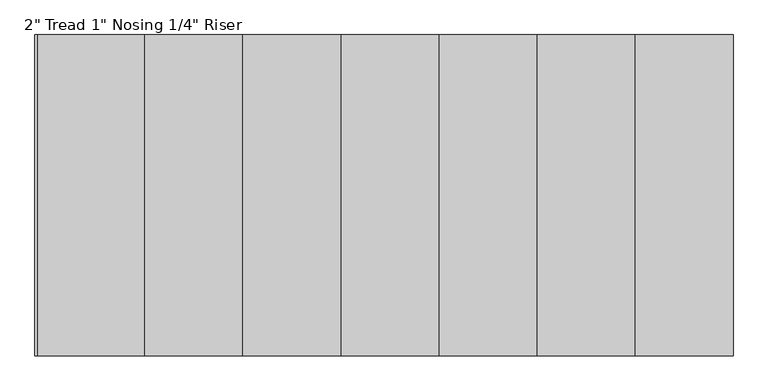
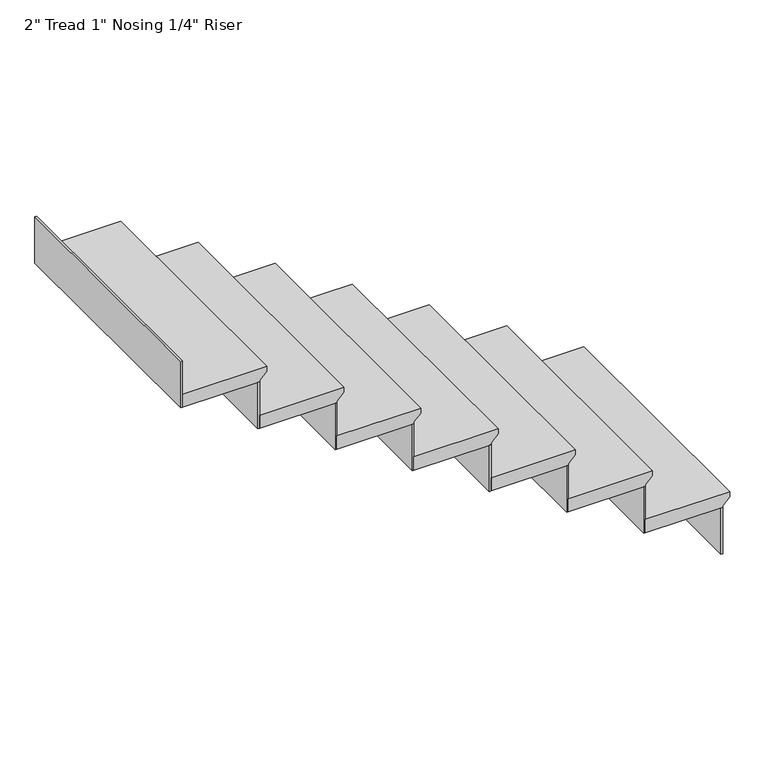
"""IFC4 building model written with IfcOpenShell, lengths in millimetres: stair flight geometry."""

from ifc_helpers import new_model, si_unit, frame, origin, place, context, project, spatial, polyline, outline, extrude, source, transform, mapped, element, save


def stair_flight_9d522be5(model_context):
    return source(origin(), model_context, "Body", "SweptSolid", [
        extrude(outline(polyline([(2565.4, -2377.5918815), (2565.4, -2682.3918815), (2514.6, -2682.3918815), (2514.6, -2402.9918815), (2520.95, -2402.9918815), (2546.35, -2377.5918815), (2565.4, -2377.5918815)])), frame((0.0, 1719.6168074, 0.0), z_axis=(0.0, 1.0, 0.0), x_axis=(0.0, 0.0, 1.0)), (0.0, 0.0, 1.0), 914.4),
        extrude(outline(polyline([(-2409.3418815, 2634.0168074), (-2402.9918815, 2634.0168074), (-2402.9918815, 1719.6168074), (-2409.3418815, 1719.6168074), (-2409.3418815, 2634.0168074)])), frame((0.0, 0.0, 2336.8), z_axis=(0.0, 0.0, 1.0), x_axis=(1.0, 0.0, 0.0)), (0.0, 0.0, 1.0), 177.8),
        extrude(outline(polyline([(-2688.7418815, 2634.0168074), (-2682.3918815, 2634.0168074), (-2682.3918815, 1719.6168074), (-2688.7418815, 1719.6168074), (-2688.7418815, 2634.0168074)])), frame((0.0, 0.0, 2514.6), z_axis=(0.0, 0.0, 1.0), x_axis=(1.0, 0.0, 0.0)), (0.0, 0.0, 1.0), 177.8),
        extrude(outline(polyline([(2743.2, -2656.9918815), (2743.2, -2961.7918815), (2692.4, -2961.7918815), (2692.4, -2682.3918815), (2698.75, -2682.3918815), (2724.15, -2656.9918815), (2743.2, -2656.9918815)])), frame((0.0, 1719.6168074, 0.0), z_axis=(0.0, 1.0, 0.0), x_axis=(0.0, 0.0, 1.0)), (0.0, 0.0, 1.0), 914.4),
        extrude(outline(polyline([(-2968.1418815, 2634.0168074), (-2961.7918815, 2634.0168074), (-2961.7918815, 1719.6168074), (-2968.1418815, 1719.6168074), (-2968.1418815, 2634.0168074)])), frame((0.0, 0.0, 2692.4), z_axis=(0.0, 0.0, 1.0), x_axis=(1.0, 0.0, 0.0)), (0.0, 0.0, 1.0), 177.8),
        extrude(outline(polyline([(2921.0, -2936.3918815), (2921.0, -3241.1918815), (2870.2, -3241.1918815), (2870.2, -2961.7918815), (2876.55, -2961.7918815), (2901.95, -2936.3918815), (2921.0, -2936.3918815)])), frame((0.0, 1719.6168074, 0.0), z_axis=(0.0, 1.0, 0.0), x_axis=(0.0, 0.0, 1.0)), (0.0, 0.0, 1.0), 914.4),
        extrude(outline(polyline([(-3247.5418815, 2634.0168074), (-3241.1918815, 2634.0168074), (-3241.1918815, 1719.6168074), (-3247.5418815, 1719.6168074), (-3247.5418815, 2634.0168074)])), frame((0.0, 0.0, 2870.2), z_axis=(0.0, 0.0, 1.0), x_axis=(1.0, 0.0, 0.0)), (0.0, 0.0, 1.0), 177.8),
        extrude(outline(polyline([(3098.8, -3215.7918815), (3098.8, -3520.5918815), (3048.0, -3520.5918815), (3048.0, -3241.1918815), (3054.35, -3241.1918815), (3079.75, -3215.7918815), (3098.8, -3215.7918815)])), frame((0.0, 1719.6168074, 0.0), z_axis=(0.0, 1.0, 0.0), x_axis=(0.0, 0.0, 1.0)), (0.0, 0.0, 1.0), 914.4),
        extrude(outline(polyline([(-3526.9418815, 2634.0168074), (-3520.5918815, 2634.0168074), (-3520.5918815, 1719.6168074), (-3526.9418815, 1719.6168074), (-3526.9418815, 2634.0168074)])), frame((0.0, 0.0, 3048.0), z_axis=(0.0, 0.0, 1.0), x_axis=(1.0, 0.0, 0.0)), (0.0, 0.0, 1.0), 177.8),
        extrude(outline(polyline([(3276.6, -3495.1918815), (3276.6, -3799.9918815), (3225.8, -3799.9918815), (3225.8, -3520.5918815), (3232.15, -3520.5918815), (3257.55, -3495.1918815), (3276.6, -3495.1918815)])), frame((0.0, 1719.6168074, 0.0), z_axis=(0.0, 1.0, 0.0), x_axis=(0.0, 0.0, 1.0)), (0.0, 0.0, 1.0), 914.4),
        extrude(outline(polyline([(-3806.3418815, 2634.0168074), (-3799.9918815, 2634.0168074), (-3799.9918815, 1719.6168074), (-3806.3418815, 1719.6168074), (-3806.3418815, 2634.0168074)])), frame((0.0, 0.0, 3225.8), z_axis=(0.0, 0.0, 1.0), x_axis=(1.0, 0.0, 0.0)), (0.0, 0.0, 1.0), 177.8),
        extrude(outline(polyline([(3454.4, -3774.5918815), (3454.4, -4079.3918815), (3403.6, -4079.3918815), (3403.6, -3799.9918815), (3409.95, -3799.9918815), (3435.35, -3774.5918815), (3454.4, -3774.5918815)])), frame((0.0, 1719.6168074, 0.0), z_axis=(0.0, 1.0, 0.0), x_axis=(0.0, 0.0, 1.0)), (0.0, 0.0, 1.0), 914.4),
        extrude(outline(polyline([(-4085.7418815, 2634.0168074), (-4079.3918815, 2634.0168074), (-4079.3918815, 1719.6168074), (-4085.7418815, 1719.6168074), (-4085.7418815, 2634.0168074)])), frame((0.0, 0.0, 3403.6), z_axis=(0.0, 0.0, 1.0), x_axis=(1.0, 0.0, 0.0)), (0.0, 0.0, 1.0), 177.8),
        extrude(outline(polyline([(-4365.1418815, 2634.0168074), (-4358.7918815, 2634.0168074), (-4358.7918815, 1719.6168074), (-4365.1418815, 1719.6168074), (-4365.1418815, 2634.0168074)])), frame((0.0, 0.0, 3581.4), z_axis=(0.0, 0.0, 1.0), x_axis=(1.0, 0.0, 0.0)), (0.0, 0.0, 1.0), 177.8),
        extrude(outline(polyline([(3632.2, -4053.9918815), (3632.2, -4358.7918815), (3581.4, -4358.7918815), (3581.4, -4079.3918815), (3587.75, -4079.3918815), (3613.15, -4053.9918815), (3632.2, -4053.9918815)])), frame((0.0, 1719.6168074, 0.0), z_axis=(0.0, 1.0, 0.0), x_axis=(0.0, 0.0, 1.0)), (0.0, 0.0, 1.0), 914.4),
    ])


if __name__ == "__main__":
    model = new_model("IFC4")
    model_context = context("Model", 3, world=origin())
    ifc_project = project(units=[si_unit("LENGTHUNIT", "METRE", prefix="MILLI")], contexts=[model_context])
    site = spatial("IfcSite", under=ifc_project)
    building = spatial("IfcBuilding", under=site)
    placement = place(None, origin())
    stair_flight_shape = stair_flight_9d522be5(model_context)
    element("IfcStairFlight", 1, ObjectType="2\" Tread 1\" Nosing 1/4\" Riser", at=placement, inside=building, context=model_context, shape_type="MappedRepresentation", body=[
        mapped(stair_flight_shape, transform((0.0, 0.0, 0.0), x_axis=(1.0, 0.0, 0.0), y_axis=(0.0, 1.0, 0.0), z_axis=(0.0, 0.0, 1.0))),
    ])
    save(model, "model.ifc")
